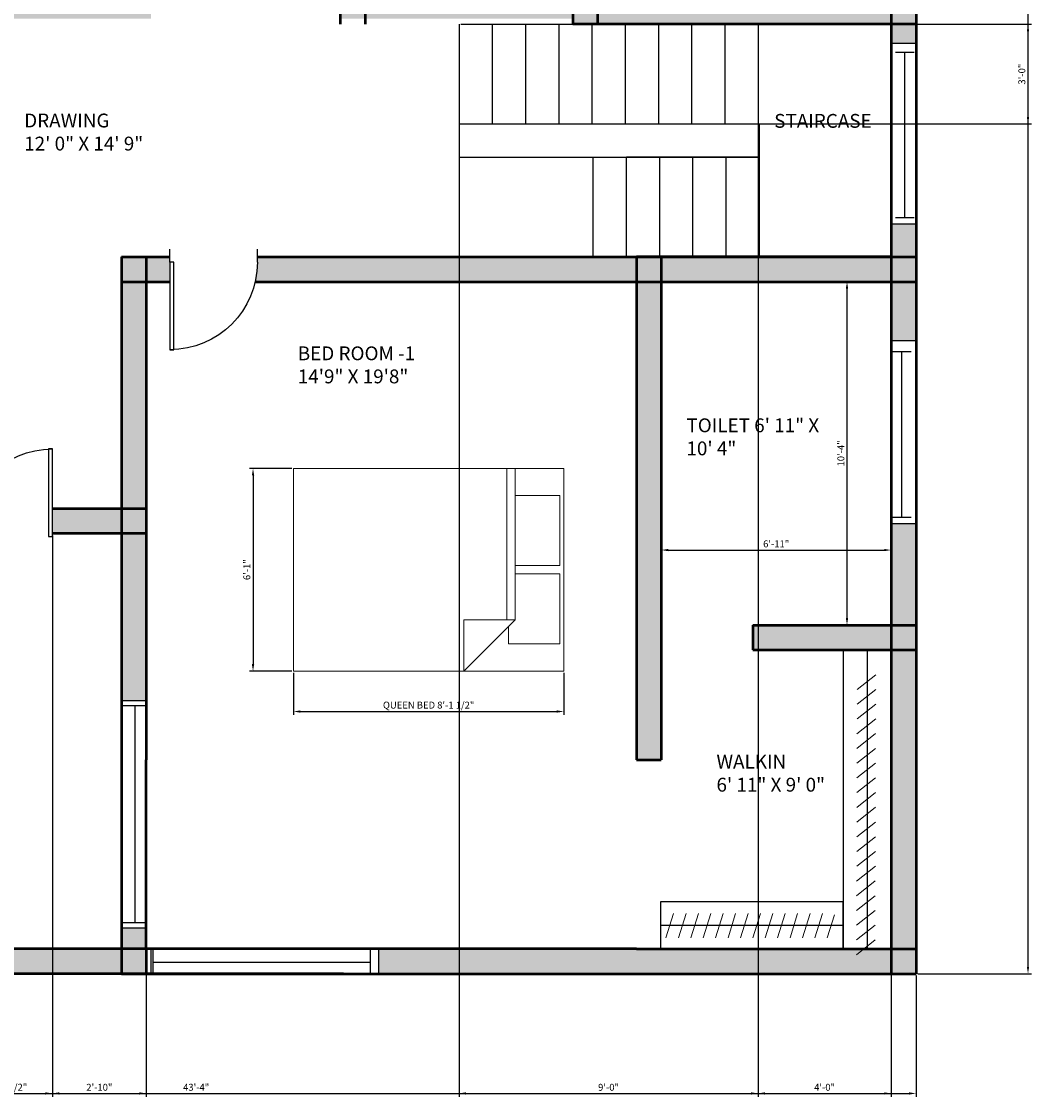
# Model space of a CAD drawing. Units: millimetres. Extents: x 2481 to 3088, y 720 to 1513.
# Tile 2 of 4: x 2723 to 3088, y 720 to 1109. Entities that reach past the tile are written whole.
import ezdxf

# ---------------------------------------------------------------- set-up
doc = ezdxf.new("R2010")
doc.units = ezdxf.units.MM
for name, color, linetype, lineweight in [('A-FLOR-CASE', 150, 'Continuous', 25), ('A-FLOR-CASE-PATT', 150, 'Continuous', 13), ('A-WALL-PATT', 5, 'Continuous', 13), ('DIMENSIONS', 10, 'Continuous', 18), ('DOORS', 213, 'Continuous', 25), ('FURNITURE', 2, 'Continuous', 18), ('STAIRCASE', 140, 'Continuous', 25), ('TEXT', 80, 'Continuous', 25), ('WALLS', 150, 'Continuous', 50), ('WINDOWS', 23, 'Continuous', 25)]:
    doc.layers.add(name, color=color, linetype=linetype, lineweight=lineweight)
doc.styles.get("Standard").update_dxf_attribs({"font": 'arial.ttf'})
doc.dimstyles.new('ISO-25', dxfattribs={"dimtxt": 2.5, "dimasz": 2.5, "dimexe": 1.25, "dimexo": 0.625, "dimtad": 1, "dimdec": 0, "dimlunit": 3, "dimtxsty": 'Standard', "dimcen": 2.5, "dimadec": 0, "dimazin": 0, "dimtfac": 1, "dimtdec": 0, "dimtmove": 0, "dimatfit": 3, "dimfxl": 1, "dimarcsym": 0})

# ---------------------------------------------------------------- blocks, each defined once
blk = doc.blocks.new('*U2')
for p, q in [((0, 0), (0, -6)), ((40, 0), (40, -6))]:
    blk.add_line(p, q)
blk.add_lwpolyline([(0, 0), (0, 40), (1.75, 40), (1.75, 0)], close=True)
blk.add_arc((0, 0), 40, 0, 90)
blk = doc.blocks.new('*U4')
for p, q in [((0, 4), (0, 0)), ((36, 4), (36, 0)), ((0, 2), (36, 2))]:
    blk.add_line(p, q)
blk = doc.blocks.new('*U5')
for p, q in [((0, 4), (0, 0)), ((36, 4), (36, 0)), ((0, 2), (36, 2))]:
    blk.add_line(p, q)
blk = doc.blocks.new('Bed - Queen')
for p, q in [((0, -80.00003), (0, 0)), ((0, 0), (59.99999, 0)), ((59.99999, 0), (59.99999, -80.00003)), ((7.99999, -1.2), (28.79998, -1.2)), ((7.99999, -14.4), (7.99999, -1.2)), ((28.79998, -1.2), (28.79998, -14.4)), ((31.19999, -1.2), (51.99999, -1.2)), ((31.19999, -14.4), (31.19999, -1.2)), ((51.99999, -1.2), (51.99999, -16.4)), ((0, -14.4), (44.8, -14.4)), ((59.99999, -29.6), (44.8, -14.4)), ((44.8, -14.4), (44.8, -29.6)), ((44.8, -16.8), (0, -16.8)), ((51.99999, -16.4), (46.79936, -16.4)), ((44.8, -29.6), (59.99999, -29.6)), ((59.99999, -80.00003), (0, -80.00003))]:
    blk.add_line(p, q)
blk = doc.blocks.new('*D25')
at = {"layer": 'Defpoints', "color": 0, "transparency": 16777216}
for p in [(2954.5, 922.47), (3037.5, 922.47), (3037.5, 918.57)]:
    blk.add_point(p, dxfattribs=at)
at = {"layer": 'DIMENSIONS', "color": 0, "lineweight": -2, "transparency": 16777216}
for p, q in [((2954.5, 921.84), (2954.5, 917.32)), ((2957, 918.57), (3035, 918.57)), ((3037.5, 921.84), (3037.5, 917.32))]:
    blk.add_line(p, q, dxfattribs=at)
at = {"layer": 'DIMENSIONS', "color": 0, "transparency": 16777216}
for points in [[(2957, 918.99), (2957, 918.16), (2954.5, 918.57)], [(3035, 918.99), (3035, 918.16), (3037.5, 918.57)]]:
    blk.add_solid(points, dxfattribs=at)
at = {"layer": 'DIMENSIONS', "color": 0, "transparency": 16777216, "insert": (2996, 920.47), "char_height": 2.5, "attachment_point": 5}
blk.add_mtext('6\'-11"', dxfattribs=at)
blk = doc.blocks.new('*D26')
at = {"layer": 'Defpoints', "color": 0, "transparency": 16777216}
for p in [(3017.06, 1015.49), (3021.58, 1015.49), (3017.06, 891.49)]:
    blk.add_point(p, dxfattribs=at)
at = {"layer": 'DIMENSIONS', "color": 0, "lineweight": -2, "transparency": 16777216}
for p, q in [((3017.69, 1015.49), (3022.83, 1015.49)), ((3021.58, 893.99), (3021.58, 1012.99)), ((3017.69, 891.49), (3022.83, 891.49))]:
    blk.add_line(p, q, dxfattribs=at)
at = {"layer": 'DIMENSIONS', "color": 0, "transparency": 16777216}
for points in [[(3021.16, 1012.99), (3021.99, 1012.99), (3021.58, 1015.49)], [(3021.16, 893.99), (3021.99, 893.99), (3021.58, 891.49)]]:
    blk.add_solid(points, dxfattribs=at)
at = {"layer": 'DIMENSIONS', "color": 0, "transparency": 16777216, "insert": (3019.68, 953.49), "char_height": 2.5, "attachment_point": 5, "rotation": 90}
blk.add_mtext('10\'-4"', dxfattribs=at)
blk = doc.blocks.new('*D35')
at = {"layer": 'Defpoints', "color": 0, "transparency": 16777216}
for p in [(2821.68, 874.88), (2919.26, 874.88), (2919.26, 860.24)]:
    blk.add_point(p, dxfattribs=at)
at = {"layer": 'DIMENSIONS', "color": 0, "lineweight": -2, "transparency": 16777216}
for p, q in [((2821.68, 874.26), (2821.68, 858.99)), ((2919.26, 874.26), (2919.26, 858.99)), ((2824.18, 860.24), (2916.76, 860.24))]:
    blk.add_line(p, q, dxfattribs=at)
at = {"layer": 'DIMENSIONS', "color": 0, "transparency": 16777216}
for points in [[(2824.18, 860.66), (2824.18, 859.83), (2821.68, 860.24)], [(2916.76, 860.66), (2916.76, 859.83), (2919.26, 860.24)]]:
    blk.add_solid(points, dxfattribs=at)
at = {"layer": 'DIMENSIONS', "color": 0, "transparency": 16777216, "insert": (2870.47, 862.24), "char_height": 2.5, "attachment_point": 5}
blk.add_mtext('QUEEN BED 8\'-1 1/2"', dxfattribs=at)
blk = doc.blocks.new('*D36')
at = {"layer": 'Defpoints', "color": 0, "transparency": 16777216}
for p in [(2821.68, 948.07), (2807.04, 874.88), (2821.68, 874.88)]:
    blk.add_point(p, dxfattribs=at)
at = {"layer": 'DIMENSIONS', "color": 0, "lineweight": -2, "transparency": 16777216}
for p, q in [((2821.05, 948.07), (2805.79, 948.07)), ((2807.04, 945.57), (2807.04, 877.38)), ((2821.05, 874.88), (2805.79, 874.88))]:
    blk.add_line(p, q, dxfattribs=at)
at = {"layer": 'DIMENSIONS', "color": 0, "transparency": 16777216}
for points in [[(2806.62, 945.57), (2807.46, 945.57), (2807.04, 948.07)], [(2806.62, 877.38), (2807.46, 877.38), (2807.04, 874.88)]]:
    blk.add_solid(points, dxfattribs=at)
at = {"layer": 'DIMENSIONS', "color": 0, "transparency": 16777216, "insert": (2805.14, 911.48), "char_height": 2.5, "attachment_point": 5, "rotation": 90}
blk.add_mtext('6\'-1"', dxfattribs=at)
blk = doc.blocks.new('*D37')
at = {"layer": 'Defpoints', "color": 0, "transparency": 16777216}
for p in [(2526.5, 765.49), (3046.5, 765.49), (3046.5, 722.28)]:
    blk.add_point(p, dxfattribs=at)
at = {"layer": 'DIMENSIONS', "color": 0, "lineweight": -2, "transparency": 16777216}
for p, q in [((2526.5, 764.86), (2526.5, 721.03)), ((3046.5, 764.86), (3046.5, 721.03)), ((2529, 722.28), (3044, 722.28))]:
    blk.add_line(p, q, dxfattribs=at)
at = {"layer": 'DIMENSIONS', "color": 0, "transparency": 16777216}
for points in [[(2529, 722.7), (2529, 721.86), (2526.5, 722.28)], [(3044, 722.7), (3044, 721.86), (3046.5, 722.28)]]:
    blk.add_solid(points, dxfattribs=at)
at = {"layer": 'DIMENSIONS', "color": 0, "transparency": 16777216, "insert": (2786.5, 724.18), "char_height": 2.5, "attachment_point": 5}
blk.add_mtext('43\'-4"', dxfattribs=at)
blk = doc.blocks.new('*D38')
at = {"layer": 'Defpoints', "color": 0, "transparency": 16777216}
for p in [(3046.5, 1473.49), (3086.95, 1473.49), (3046.5, 765.49)]:
    blk.add_point(p, dxfattribs=at)
at = {"layer": 'DIMENSIONS', "color": 0, "lineweight": -2, "transparency": 16777216}
for p, q in [((3047.12, 1473.49), (3088.2, 1473.49)), ((3086.95, 767.99), (3086.95, 1470.99)), ((3047.12, 765.49), (3088.2, 765.49))]:
    blk.add_line(p, q, dxfattribs=at)
at = {"layer": 'DIMENSIONS', "color": 0, "transparency": 16777216}
for points in [[(3086.53, 1470.99), (3087.36, 1470.99), (3086.95, 1473.49)], [(3086.53, 767.99), (3087.36, 767.99), (3086.95, 765.49)]]:
    blk.add_solid(points, dxfattribs=at)
at = {"layer": 'DIMENSIONS', "color": 0, "transparency": 16777216, "insert": (3085.04, 1119.49), "char_height": 2.5, "attachment_point": 5, "rotation": 90}
blk.add_mtext('59\'-0"', dxfattribs=at)
blk = doc.blocks.new('*D42')
at = {"layer": 'Defpoints', "color": 0, "transparency": 16777216}
for p in [(2881.45, 1072.49), (2989.45, 1072.49), (2989.45, 722.28)]:
    blk.add_point(p, dxfattribs=at)
at = {"layer": 'DIMENSIONS', "color": 0, "lineweight": -2, "transparency": 16777216}
for p, q in [((2881.45, 1071.86), (2881.45, 721.03)), ((2989.45, 1071.86), (2989.45, 721.03)), ((2883.95, 722.28), (2986.95, 722.28))]:
    blk.add_line(p, q, dxfattribs=at)
at = {"layer": 'DIMENSIONS', "color": 0, "transparency": 16777216}
for points in [[(2883.95, 722.7), (2883.95, 721.86), (2881.45, 722.28)], [(2986.95, 722.7), (2986.95, 721.86), (2989.45, 722.28)]]:
    blk.add_solid(points, dxfattribs=at)
at = {"layer": 'DIMENSIONS', "color": 0, "transparency": 16777216, "insert": (2935.45, 724.18), "char_height": 2.5, "attachment_point": 5}
blk.add_mtext('9\'-0"', dxfattribs=at)
blk = doc.blocks.new('*D43')
at = {"layer": 'Defpoints', "color": 0, "transparency": 16777216}
for p in [(2881.45, 1108.49), (3086.95, 1108.49), (2881.45, 1072.49)]:
    blk.add_point(p, dxfattribs=at)
at = {"layer": 'DIMENSIONS', "color": 0, "lineweight": -2, "transparency": 16777216}
for p, q in [((2882.08, 1108.49), (3088.2, 1108.49)), ((3086.95, 1074.99), (3086.95, 1105.99)), ((2882.08, 1072.49), (3088.2, 1072.49))]:
    blk.add_line(p, q, dxfattribs=at)
at = {"layer": 'DIMENSIONS', "color": 0, "transparency": 16777216}
for points in [[(3086.53, 1105.99), (3087.36, 1105.99), (3086.95, 1108.49)], [(3086.53, 1074.99), (3087.36, 1074.99), (3086.95, 1072.49)]]:
    blk.add_solid(points, dxfattribs=at)
at = {"layer": 'DIMENSIONS', "color": 0, "transparency": 16777216, "insert": (3085.04, 1090.49), "char_height": 2.5, "attachment_point": 5, "rotation": 90}
blk.add_mtext('3\'-0"', dxfattribs=at)
blk = doc.blocks.new('*D44')
at = {"layer": 'Defpoints', "color": 0, "transparency": 16777216}
for p in [(2989.45, 1108.49), (3037.5, 1101.52), (3037.5, 722.28)]:
    blk.add_point(p, dxfattribs=at)
at = {"layer": 'DIMENSIONS', "color": 0, "lineweight": -2, "transparency": 16777216}
for p, q in [((2989.45, 1107.86), (2989.45, 721.03)), ((3037.5, 1100.89), (3037.5, 721.03)), ((2991.95, 722.28), (3035, 722.28))]:
    blk.add_line(p, q, dxfattribs=at)
at = {"layer": 'DIMENSIONS', "color": 0, "transparency": 16777216}
for points in [[(2991.95, 722.7), (2991.95, 721.86), (2989.45, 722.28)], [(3035, 722.7), (3035, 721.86), (3037.5, 722.28)]]:
    blk.add_solid(points, dxfattribs=at)
at = {"layer": 'DIMENSIONS', "color": 0, "transparency": 16777216, "insert": (3013.48, 724.18), "char_height": 2.5, "attachment_point": 5}
blk.add_mtext('4\'-0"', dxfattribs=at)
blk = doc.blocks.new('*D45')
at = {"layer": 'Defpoints', "color": 0, "transparency": 16777216}
for p in [(2703, 924.49), (2734.57, 924.49), (2734.57, 722.28)]:
    blk.add_point(p, dxfattribs=at)
at = {"layer": 'DIMENSIONS', "color": 0, "lineweight": -2, "transparency": 16777216}
for p, q in [((2703, 923.86), (2703, 721.03)), ((2734.57, 923.86), (2734.57, 721.03)), ((2705.5, 722.28), (2732.07, 722.28))]:
    blk.add_line(p, q, dxfattribs=at)
at = {"layer": 'DIMENSIONS', "color": 0, "transparency": 16777216}
for points in [[(2705.5, 722.7), (2705.5, 721.86), (2703, 722.28)], [(2732.07, 722.7), (2732.07, 721.86), (2734.57, 722.28)]]:
    blk.add_solid(points, dxfattribs=at)
at = {"layer": 'DIMENSIONS', "color": 0, "transparency": 16777216, "insert": (2718.78, 724.2), "char_height": 2.5, "attachment_point": 5}
blk.add_mtext('2\'-7 1/2"', dxfattribs=at)
blk = doc.blocks.new('*D46')
at = {"layer": 'Defpoints', "color": 0, "transparency": 16777216}
for p in [(2734.57, 924.49), (2768.5, 924.49), (2768.5, 722.28)]:
    blk.add_point(p, dxfattribs=at)
at = {"layer": 'DIMENSIONS', "color": 0, "lineweight": -2, "transparency": 16777216}
for p, q in [((2734.57, 923.86), (2734.57, 721.03)), ((2768.5, 923.86), (2768.5, 721.03)), ((2737.07, 722.28), (2766, 722.28))]:
    blk.add_line(p, q, dxfattribs=at)
at = {"layer": 'DIMENSIONS', "color": 0, "transparency": 16777216}
for points in [[(2737.07, 722.7), (2737.07, 721.86), (2734.57, 722.28)], [(2766, 722.7), (2766, 721.86), (2768.5, 722.28)]]:
    blk.add_solid(points, dxfattribs=at)
at = {"layer": 'DIMENSIONS', "color": 0, "transparency": 16777216, "insert": (2751.53, 724.18), "char_height": 2.5, "attachment_point": 5}
blk.add_mtext('2\'-10"', dxfattribs=at)

msp = doc.modelspace()

# ---------------------------------------------------------------- hatches: boundary and pattern name
at = {"layer": 'A-FLOR-CASE-PATT'}
h = msp.add_hatch(dxfattribs=at)
h.set_pattern_fill('ANSI31', color=256, scale=1.312577, angle=-6.652, style=0)
h.paths.add_polyline_path([(3025, 771.45), (3031.75, 776.8), (3031.78, 787.44), (3031.85, 819.38), (3031.89, 840.67), (3031.92, 851.32), (3031.93, 856.64), (3031.97, 877.93), (3025.22, 872.59), (3025.17, 851.3), (3025.1, 819.36)])
h = msp.add_hatch(dxfattribs=at)
h.set_pattern_fill('ANSI31', color=256, scale=1.34533, angle=27.463, style=0)
h.paths.add_polyline_path([(2955.37, 778.52), (3018.09, 778.52), (3020.17, 785.09), (3016.37, 787.25), (2958.13, 787.25)])
at = {"layer": 'A-WALL-PATT'}
h = msp.add_hatch(color=256, dxfattribs=at)
h.dxf.hatch_style = 1
h.paths.add_polyline_path([(2599.5, 1473.49), (2590.5, 1473.49), (2590.5, 1464.49), (2599.5, 1464.49)])
h.paths.add_polyline_path([(2599.5, 1464.49), (2590.5, 1464.49), (2590.5, 1447.8), (2599.5, 1447.8)])
h.paths.add_polyline_path([(2625.38, 1473.49), (2599.5, 1473.49), (2599.5, 1464.49), (2625.38, 1464.49)])
h.paths.add_polyline_path([(2805.36, 1473.49), (2710.95, 1473.49), (2710.95, 1464.49), (2805.36, 1464.49)])
h.paths.add_polyline_path([(2922.5, 1473.49), (2830.18, 1473.49), (2830.18, 1464.49), (2922.5, 1464.49)])
h.paths.add_polyline_path([(2931.5, 1473.49), (2922.5, 1473.49), (2922.5, 1464.49), (2931.5, 1464.49)])
h.paths.add_polyline_path([(2931.5, 1464.49), (2922.5, 1464.49), (2922.5, 1402.56), (2926.01, 1402.56, -0.043673), (2931.5, 1402.08)])
h.paths.add_polyline_path([(2931.5, 1368.49), (2922.5, 1368.49), (2922.5, 1359.49), (2931.5, 1359.49)])
h.paths.add_polyline_path([(2922.5, 1296.49), (2675.15, 1296.49), (2675.15, 1287.49), (2922.5, 1287.49)])
h.paths.add_polyline_path([(2931.5, 1294.49), (2922.5, 1294.49), (2922.5, 1287.49), (2922.5, 1285.49), (2931.5, 1285.49)])
h.paths.add_polyline_path([(3037.5, 1294.49), (2931.5, 1294.49), (2931.5, 1285.49), (3037.5, 1285.49)])
h.paths.add_polyline_path([(3046.5, 1294.49), (3037.5, 1294.49), (3037.5, 1285.49), (3046.5, 1285.49)])
h.paths.add_polyline_path([(3046.5, 1316.66), (3037.5, 1316.66), (3037.5, 1294.49), (3046.5, 1294.49)])
h.paths.add_polyline_path([(3046.5, 1359.49), (3037.5, 1359.49), (3037.5, 1343.26), (3046.5, 1343.26)])
h.paths.add_polyline_path([(3046.5, 1368.49), (3037.5, 1368.49), (3037.5, 1359.49), (3046.5, 1359.49)])
h.paths.add_polyline_path([(3037.5, 1368.49), (2931.5, 1368.49), (2931.5, 1359.49), (3037.5, 1359.49)])
h.paths.add_polyline_path([(2599.5, 1361.25), (2590.5, 1361.25), (2590.5, 1233.6), (2599.5, 1233.6)])
h.paths.add_polyline_path([(2535.5, 1110.49), (2526.5, 1110.49), (2526.5, 933.49), (2535.5, 933.49)])
h.paths.add_polyline_path([(2535.5, 1119.49), (2526.5, 1119.49), (2526.5, 1110.49), (2535.5, 1110.49)])
h.paths.add_polyline_path([(2590.5, 1119.49), (2535.5, 1119.49), (2535.5, 1110.49), (2590.5, 1110.49)])
h.paths.add_polyline_path([(2599.5, 1119.49), (2594.5, 1119.49), (2590.5, 1119.49), (2590.5, 1110.49), (2594.5, 1110.49), (2599.5, 1110.49)])
h.paths.add_polyline_path([(2599.5, 1148.41), (2590.5, 1148.41), (2590.5, 1119.49), (2594.5, 1119.49), (2599.5, 1119.49)])
h.paths.add_polyline_path([(2770.14, 1119.49), (2599.5, 1119.49), (2599.5, 1110.49), (2770.14, 1110.49)])
h.paths.add_polyline_path([(3037.5, 1473.49), (2931.5, 1473.49), (2931.5, 1464.49), (3037.5, 1464.49)])
h.paths.add_polyline_path([(3046.5, 1473.49), (3037.5, 1473.49), (3037.5, 1464.49), (3046.5, 1464.49)])
h.paths.add_polyline_path([(2535.5, 842.83), (2535.5, 924.49), (2526.5, 924.49), (2526.5, 774.49), (2535.5, 774.49)])
h.paths.add_polyline_path([(2535.5, 774.49), (2526.5, 774.49), (2526.5, 765.49), (2535.5, 765.49)])
h.paths.add_polyline_path([(3037.5, 774.49), (2945.5, 774.49), (2852.34, 774.49), (2852.34, 765.49), (3037.5, 765.49)])
h.paths.add_polyline_path([(3046.5, 774.49), (3037.5, 774.49), (3037.5, 765.49), (3046.5, 765.49)])
h.paths.add_polyline_path([(3046.5, 882.49), (3037.5, 882.49), (3037.5, 774.49), (3046.5, 774.49)])
h.paths.add_polyline_path([(2768.5, 774.49), (2759.5, 774.49), (2759.5, 765.49), (2768.5, 765.49)])
h.paths.add_polyline_path([(2759.5, 774.49), (2535.5, 774.49), (2535.5, 765.49), (2759.5, 765.49)])
h.paths.add_polyline_path([(2768.5, 781.94), (2759.5, 781.94), (2759.5, 774.49), (2768.5, 774.49)])
h.paths.add_polyline_path([(2768.5, 1015.49), (2759.5, 1015.49), (2759.5, 933.49), (2768.5, 933.49)])
h.paths.add_polyline_path([(2768.5, 933.49), (2759.5, 933.49), (2759.5, 924.49), (2768.5, 924.49)])
h.paths.add_polyline_path([(2768.5, 924.49), (2759.5, 924.49), (2759.5, 864.16), (2768.5, 864.16)])
h.paths.add_polyline_path([(2759.5, 933.49), (2734.57, 933.49), (2734.57, 924.49), (2759.5, 924.49)])
h.paths.add_polyline_path([(2954.5, 1015.49), (2945.5, 1015.49), (2945.5, 842.83), (2954.5, 842.83)])
h.paths.add_polyline_path([(2954.5, 1024.49), (2945.5, 1024.49), (2945.5, 1015.49), (2954.5, 1015.49)])
h.paths.add_polyline_path([(2945.5, 1024.49), (2808.62, 1024.49), (2808.62, 1022.52, -0.056199), (2807.82, 1015.49), (2945.5, 1015.49)])
h.paths.add_polyline_path([(3037.5, 1024.49), (2954.5, 1024.49), (2954.5, 1015.49), (3037.5, 1015.49)])
h.paths.add_polyline_path([(3046.5, 1024.49), (3037.5, 1024.49), (3037.5, 1015.49), (3046.5, 1015.49)])
h.paths.add_polyline_path([(3046.5, 1015.49), (3037.5, 1015.49), (3037.5, 994.13), (3046.5, 994.13)])
h.paths.add_polyline_path([(3046.5, 928.1), (3037.5, 928.1), (3037.5, 891.49), (3046.5, 891.49)])
h.paths.add_polyline_path([(3046.5, 891.49), (3037.5, 891.49), (3037.5, 882.49), (3046.5, 882.49)])
h.paths.add_polyline_path([(3037.5, 891.49), (2987.62, 891.49), (2987.62, 882.49), (3037.5, 882.49)])
h.paths.add_polyline_path([(2768.5, 1024.49), (2759.5, 1024.49), (2759.5, 1015.49), (2768.5, 1015.49)])
h.paths.add_polyline_path([(2777.03, 1022.52), (2777.03, 1024.49), (2768.5, 1024.49), (2768.5, 1015.49), (2777.03, 1015.49)])
h = msp.add_hatch(color=256, dxfattribs=at)
h.dxf.hatch_style = 1
h.paths.add_polyline_path([(2931.5, 1211.49), (2922.5, 1211.49), (2922.5, 1117.49), (2931.5, 1117.49)])
h.paths.add_polyline_path([(2931.5, 1285.49), (2922.5, 1285.49), (2922.5, 1220.49), (2931.5, 1220.49)])
h.paths.add_polyline_path([(2931.5, 1325.63), (2922.5, 1325.63), (2922.5, 1294.49), (2931.5, 1294.49)])
h.paths.add_polyline_path([(2869.83, 1270.23), (2869.83, 1287.49), (2860.83, 1287.49), (2860.83, 1270.23), (2838.5, 1270.23), (2838.5, 1261.23), (2860.83, 1261.23), (2869.83, 1261.23)])
h.paths.add_polyline_path([(3037.5, 1220.49), (2931.5, 1220.49), (2931.5, 1211.49), (3037.5, 1211.49)])
h.paths.add_polyline_path([(2931.5, 1220.49), (2922.5, 1220.49), (2922.5, 1211.49), (2931.5, 1211.49)])
h.paths.add_polyline_path([(3046.5, 1220.49), (3037.5, 1220.49), (3037.5, 1211.49), (3046.5, 1211.49)])
h.paths.add_polyline_path([(3046.5, 1252.04), (3046.4, 1252.04, -0.071368), (3037.5, 1253.12), (3037.5, 1220.49), (3046.5, 1220.49)])
h.paths.add_polyline_path([(2847.5, 1193.49), (2838.5, 1193.49), (2838.5, 1184.49), (2847.5, 1184.49)])
h.paths.add_polyline_path([(2922.5, 1193.49), (2847.5, 1193.49), (2847.5, 1184.49), (2922.5, 1184.49)])
h.paths.add_polyline_path([(2847.5, 1229.29), (2838.5, 1229.29), (2838.5, 1193.49), (2847.5, 1193.49)])
h.paths.add_polyline_path([(2847.5, 1184.49), (2838.5, 1184.49), (2838.5, 1119.49), (2847.5, 1119.49)])
h.paths.add_polyline_path([(2922.5, 1119.49), (2847.5, 1119.49), (2847.5, 1110.49), (2922.5, 1110.49)])
h.paths.add_polyline_path([(2847.5, 1119.49), (2838.5, 1119.49), (2838.5, 1110.49), (2847.5, 1110.49)])
h.paths.add_polyline_path([(3037.5, 1117.49), (2931.5, 1117.49), (2931.5, 1108.49), (3037.5, 1108.49)])
h.paths.add_polyline_path([(2931.5, 1117.49), (2922.5, 1117.49), (2922.5, 1110.49), (2922.5, 1108.49), (2931.5, 1108.49)])
h.paths.add_polyline_path([(3046.5, 1117.49), (3037.5, 1117.49), (3037.5, 1108.49), (3046.5, 1108.49)])
h.paths.add_polyline_path([(3046.5, 1176.98), (3045.26, 1176.98, -0.062137), (3037.5, 1177.95), (3037.5, 1117.49), (3046.5, 1117.49)])
h.paths.add_polyline_path([(3046.5, 1108.49), (3037.5, 1108.49), (3037.5, 1101.52), (3046.5, 1101.52)])
h.paths.add_polyline_path([(3046.5, 1024.49), (3037.5, 1024.49), (3037.5, 1015.49), (3046.5, 1015.49)])
h.paths.add_polyline_path([(3046.5, 1036.41), (3037.5, 1036.41), (3037.5, 1024.49), (3046.5, 1024.49)])

# ---------------------------------------------------------------- linework, layer by layer
at = {"layer": 'A-FLOR-CASE'}
for p, q in [((3037.5, 882.49), (3020.17, 882.49)), ((3020.17, 882.49), (3020.17, 774.49)), ((3028.83, 882.49), (3028.83, 774.49)), ((3020.17, 791.54), (2954.18, 791.54)), ((2954.18, 791.54), (2954.18, 774.49)), ((3020.17, 774.49), (3020.17, 791.54)), ((2954.18, 783.01), (3020.17, 783.01))]:
    msp.add_line(p, q, dxfattribs=at)
at = {"layer": 'STAIRCASE'}
for p, q in [((2881.45, 1108.49), (2881.45, 1072.49)), ((2893.45, 1108.49), (2893.45, 1072.49)), ((2905.45, 1108.49), (2905.45, 1072.49)), ((2917.45, 1108.49), (2917.45, 1072.49)), ((2929.45, 1108.49), (2929.45, 1072.49)), ((2941.45, 1108.49), (2941.45, 1072.49)), ((2953.45, 1108.49), (2953.45, 1072.49)), ((2965.45, 1108.49), (2965.45, 1072.49)), ((2977.45, 1108.49), (2977.45, 1072.49)), ((2989.45, 1108.49), (2989.45, 1072.49)), ((2881.45, 1072.49), (2989.45, 1072.49)), ((2881.45, 1072.49), (2881.45, 1060.49)), ((2989.92, 1072.47), (2989.45, 1072.49)), ((2989.92, 1060.49), (2989.92, 1072.47)), ((2881.45, 1060.49), (2989.92, 1060.49)), ((2929.92, 1024.49), (2929.92, 1060.49)), ((2941.92, 1024.49), (2941.92, 1060.49)), ((2989.92, 1060.49), (2941.92, 1060.49)), ((2953.92, 1024.49), (2953.92, 1060.49)), ((2965.92, 1024.49), (2965.92, 1060.49)), ((2977.92, 1024.49), (2977.92, 1060.49)), ((2989.92, 1024.49), (2989.92, 1060.49))]:
    msp.add_line(p, q, dxfattribs=at)
at = {"layer": 'WALLS'}
for p, q in [((2922.5, 1325.63), (2922.5, 1108.49)), ((2931.5, 1325.63), (2931.5, 1108.49)), ((2838.5, 1229.29), (2838.5, 1108.49)), ((2847.5, 1229.29), (2847.5, 1108.49)), ((3037.5, 1177.95), (3037.5, 765.49)), ((3046.5, 1176.98), (3046.5, 765.49)), ((3046.5, 1108.49), (2922.5, 1108.49)), ((2759.5, 1024.49), (2777.03, 1024.49)), ((2759.5, 1024.49), (2759.5, 842.83)), ((2768.5, 1024.49), (2768.5, 842.83)), ((2808.62, 1024.49), (3046.5, 1024.49)), ((2954.5, 1024.49), (2945.5, 1024.49)), ((2945.5, 1024.49), (2945.5, 842.83)), ((3037.5, 1024.49), (2954.5, 1024.49)), ((2954.5, 1024.49), (2954.5, 842.83)), ((2992.44, 1024.49), (3037.5, 1024.49)), ((2759.5, 1015.49), (2777.03, 1015.49)), ((2807.82, 1015.49), (3046.5, 1015.49)), ((2768.5, 933.49), (2734.57, 933.49)), ((2768.5, 924.49), (2734.57, 924.49)), ((2987.62, 891.49), (2987.62, 882.49)), ((2987.62, 891.49), (3046.5, 891.49)), ((2987.62, 882.49), (3046.5, 882.49)), ((2759.5, 842.83), (2759.5, 765.49)), ((2768.5, 774.49), (2768.5, 842.83)), ((2945.5, 842.83), (2954.5, 842.83)), ((2839.77, 774.49), (2526.5, 774.49)), ((2768.5, 774.49), (2768.5, 765.49)), ((2945.5, 774.49), (2839.77, 774.49)), ((2945.5, 774.49), (3046.5, 774.49)), ((2839.77, 765.49), (2526.5, 765.49)), ((2759.5, 765.49), (2768.5, 765.49)), ((2768.5, 765.49), (3046.5, 765.49))]:
    msp.add_line(p, q, dxfattribs=at)
at = {"layer": 'WINDOWS'}
for p, q in [((3046.5, 1101.52), (3037.5, 1101.52)), ((3037.5, 1036.41), (3046.5, 1036.41)), ((3046.5, 994.13), (3037.5, 994.13)), ((3046.5, 928.1), (3037.5, 928.1)), ((2768.5, 864.16), (2759.5, 864.16)), ((2768.5, 781.94), (2759.5, 781.94)), ((2770.16, 774.49), (2770.16, 765.49)), ((2852.34, 774.49), (2852.34, 765.49))]:
    msp.add_line(p, q, dxfattribs=at)

# ---------------------------------------------------------------- block references
at = {"layer": 'DOORS', "xscale": -0.7896024204950681, "yscale": 0.7896024204950681, "zscale": 0.7896024204950681}
for p, rotation in [((2777.03, 1022.52), 180), ((2734.57, 923.5), 359.9999960046612)]:
    msp.add_blockref('*U2', p, dxfattribs=dict(at, rotation=rotation))
at = {"layer": 'FURNITURE', "xscale": 1.219827458287992, "yscale": 1.219827458287992, "zscale": 1.219827458287992, "rotation": 269.9999999999995}
msp.add_blockref('Bed - Queen', (2919.26, 948.07), dxfattribs=at)
at = {"layer": 'WINDOWS', "rotation": 90}
for name, p, xscale, yscale, zscale in [('*U5', (3045.78, 1038.67), 1.660051456791394, 1.660051456791394, 1.660051456791394), ('*U5', (3044.74, 930.5), 1.660051456791394, 1.660051456791394, 1.660051456791394), ('*U4', (2768.86, 784), 2.179725659021641, 2.179725659021641, 2.179725659021641)]:
    msp.add_blockref(name, p, dxfattribs=dict(at, xscale=xscale, yscale=yscale, zscale=zscale))
at = {"layer": 'WINDOWS', "xscale": 2.179725659021641, "yscale": 2.179725659021641, "zscale": 2.179725659021641}
msp.add_blockref('*U4', (2770.89, 765.34), dxfattribs=at)

# ---------------------------------------------------------------- texts
at = {"layer": 'TEXT', "char_height": 5, "attachment_point": 1}
for s, width, insert in [('DRAWING \\P12\' 0" X 14\' 9"', 67.7142, (2724.39, 1076.23)), ('STAIRCASE', 37.9162, (2995.28, 1076.1)), ('BED ROOM -1 \\P14\'9" X 19\'8"', 112.1821, (2823.2, 992.13)), ('TOILET 6\' 11" X 10\' 4"', 52.0242, (2963.58, 966.13)), ('WALKIN \\P6\' 11" X 9\' 0"', 51.0263, (2974.43, 844.64))]:
    msp.add_mtext_dynamic_manual_height_columns(s, width=width, gutter_width=12.5, heights=[0], dxfattribs=dict(at, insert=insert))

# ---------------------------------------------------------------- dimensions: what is measured, and where the dimension line sits
at = {"layer": 'DIMENSIONS'}
for base, p1, p2, angle, override, picture, middle in [((3086.95, 1473.49), (3046.5, 765.49), (3046.5, 1473.49), 90, {"dimdec": 1, "dimlfac": 1, "dimrnd": 0, "dimzin": 1, "dimdsep": 46, "dimlunit": 4, "dimfrac": 2}, '*D38', (3085.04, 1119.49)), ((3086.95, 1108.49), (2881.45, 1072.49), (2881.45, 1108.49), 90, {"dimdec": 1, "dimlfac": 1, "dimrnd": 0, "dimzin": 1, "dimdsep": 46, "dimlunit": 4, "dimfrac": 2}, '*D43', (3085.04, 1090.49)), ((3021.58, 1015.49), (3017.06, 891.49), (3017.06, 1015.49), 90, {"dimclrd": 0, "dimclre": 0, "dimclrt": 0}, '*D26', (3019.68, 953.49)), ((2807.04, 874.88), (2821.68, 948.07), (2821.68, 874.88), 270, {"dimdec": 1, "dimlfac": 1, "dimrnd": 0, "dimzin": 1, "dimdsep": 46, "dimlunit": 4, "dimfrac": 2}, '*D36', (2805.14, 911.48))]:
    dim = msp.add_linear_dim(base=base, p1=p1, p2=p2, angle=angle, dimstyle='ISO-25', override=override, dxfattribs=at)
    dim.commit()
    dim.dimension.update_dxf_attribs({"geometry": picture, "text_midpoint": middle})
for base, p1, p2, override, picture, middle in [((3037.4994, 722.2785), (2989.4517, 1108.4867), (3037.4994, 1101.5195), {"dimdec": 1, "dimlfac": 1, "dimrnd": 0, "dimzin": 1, "dimdsep": 46, "dimlunit": 4, "dimfrac": 2}, '*D44', (3013.4755, 724.1799)), ((2989.45, 722.28), (2881.45, 1072.49), (2989.45, 1072.49), {"dimdec": 1, "dimlfac": 1, "dimrnd": 0, "dimzin": 1, "dimdsep": 46, "dimlunit": 4, "dimfrac": 2}, '*D42', (2935.45, 724.18)), ((2734.57, 722.28), (2703, 924.49), (2734.57, 924.49), {"dimdec": 1, "dimlfac": 1, "dimrnd": 0, "dimzin": 1, "dimdsep": 46, "dimlunit": 4, "dimfrac": 2}, '*D45', (2718.78, 724.2)), ((2768.5, 722.28), (2734.57, 924.49), (2768.5, 924.49), {"dimdec": 1, "dimlfac": 1, "dimrnd": 0, "dimzin": 1, "dimdsep": 46, "dimlunit": 4, "dimfrac": 2}, '*D46', (2751.53, 724.18)), ((3037.5, 918.57), (2954.5, 922.47), (3037.5, 922.47), {"dimclrd": 0, "dimclre": 0, "dimclrt": 0}, '*D25', (2996, 920.47)), ((3046.5, 722.28), (2526.5, 765.49), (3046.5, 765.49), {"dimdec": 1, "dimlfac": 1, "dimrnd": 0, "dimzin": 1, "dimdsep": 46, "dimlunit": 4, "dimfrac": 2}, '*D37', (2786.5, 724.18))]:
    dim = msp.add_linear_dim(base=base, p1=p1, p2=p2, dimstyle='ISO-25', override=override, dxfattribs=at)
    dim.commit()
    dim.dimension.update_dxf_attribs({"geometry": picture, "text_midpoint": middle})
dim = msp.add_linear_dim(base=(2919.26, 860.24), p1=(2821.68, 874.88), p2=(2919.26, 874.88), text='QUEEN BED <>', dimstyle='ISO-25', override={"dimdec": 1, "dimlfac": 1, "dimrnd": 0, "dimzin": 1, "dimdsep": 46, "dimlunit": 4, "dimfrac": 2}, dxfattribs=at)
dim.commit()
dim.dimension.update_dxf_attribs({"geometry": '*D35', "text_midpoint": (2870.47, 862.24)})

doc.saveas('drawing.dxf')
